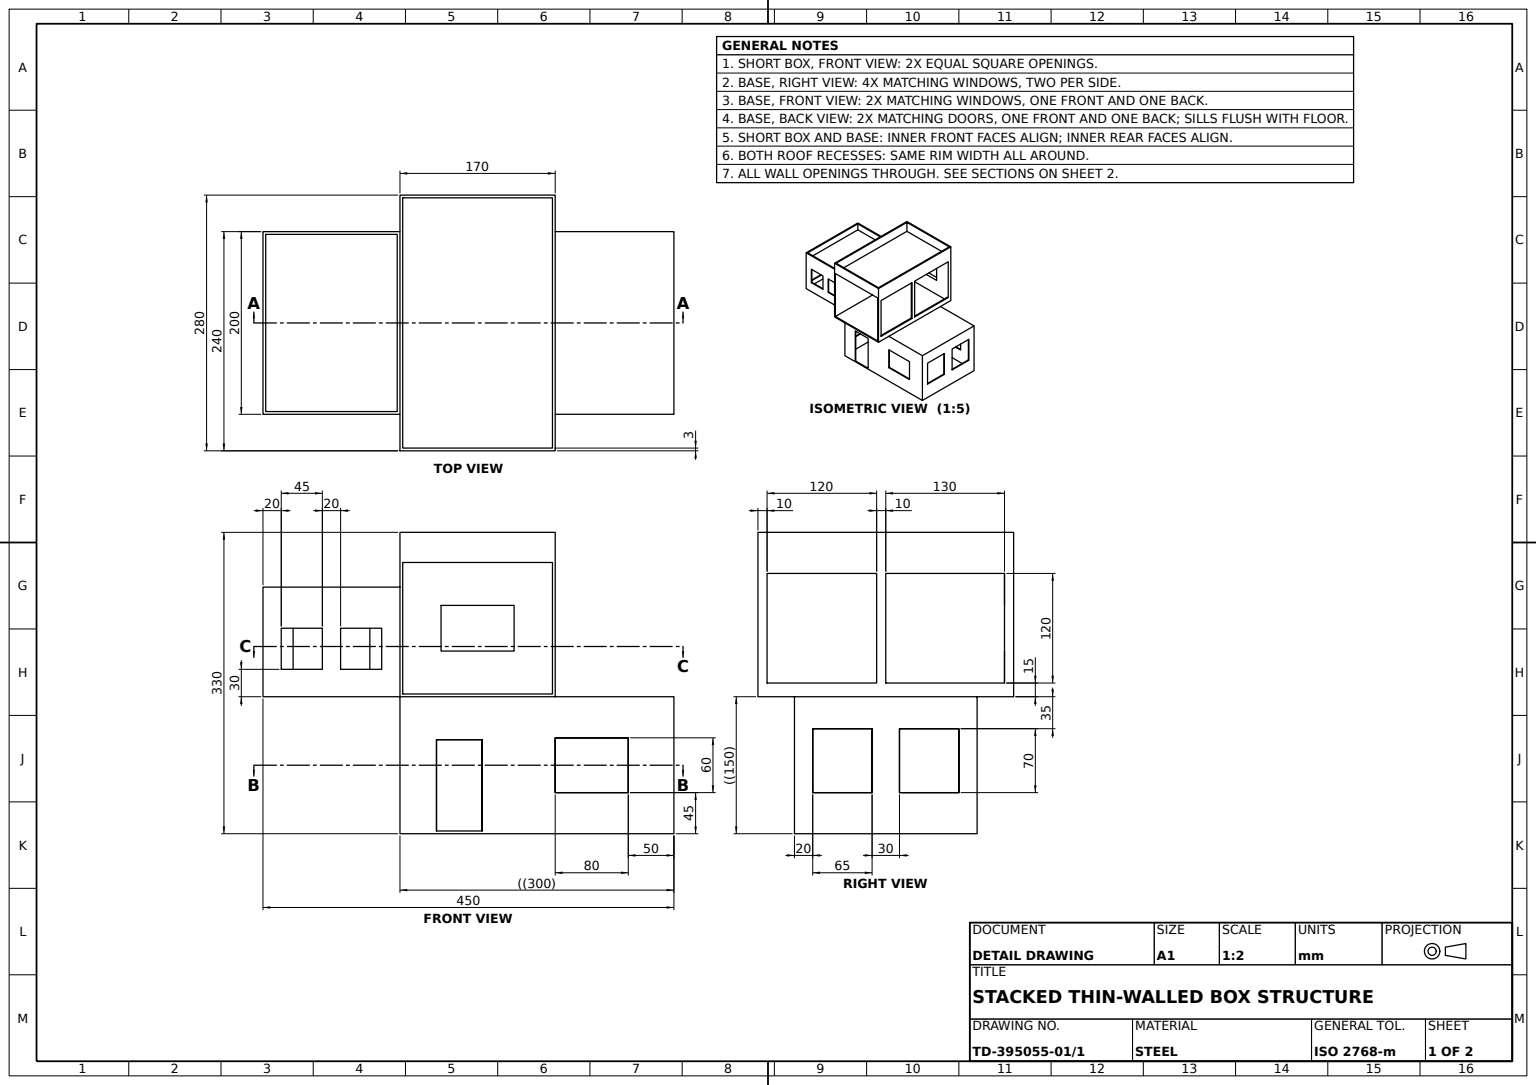
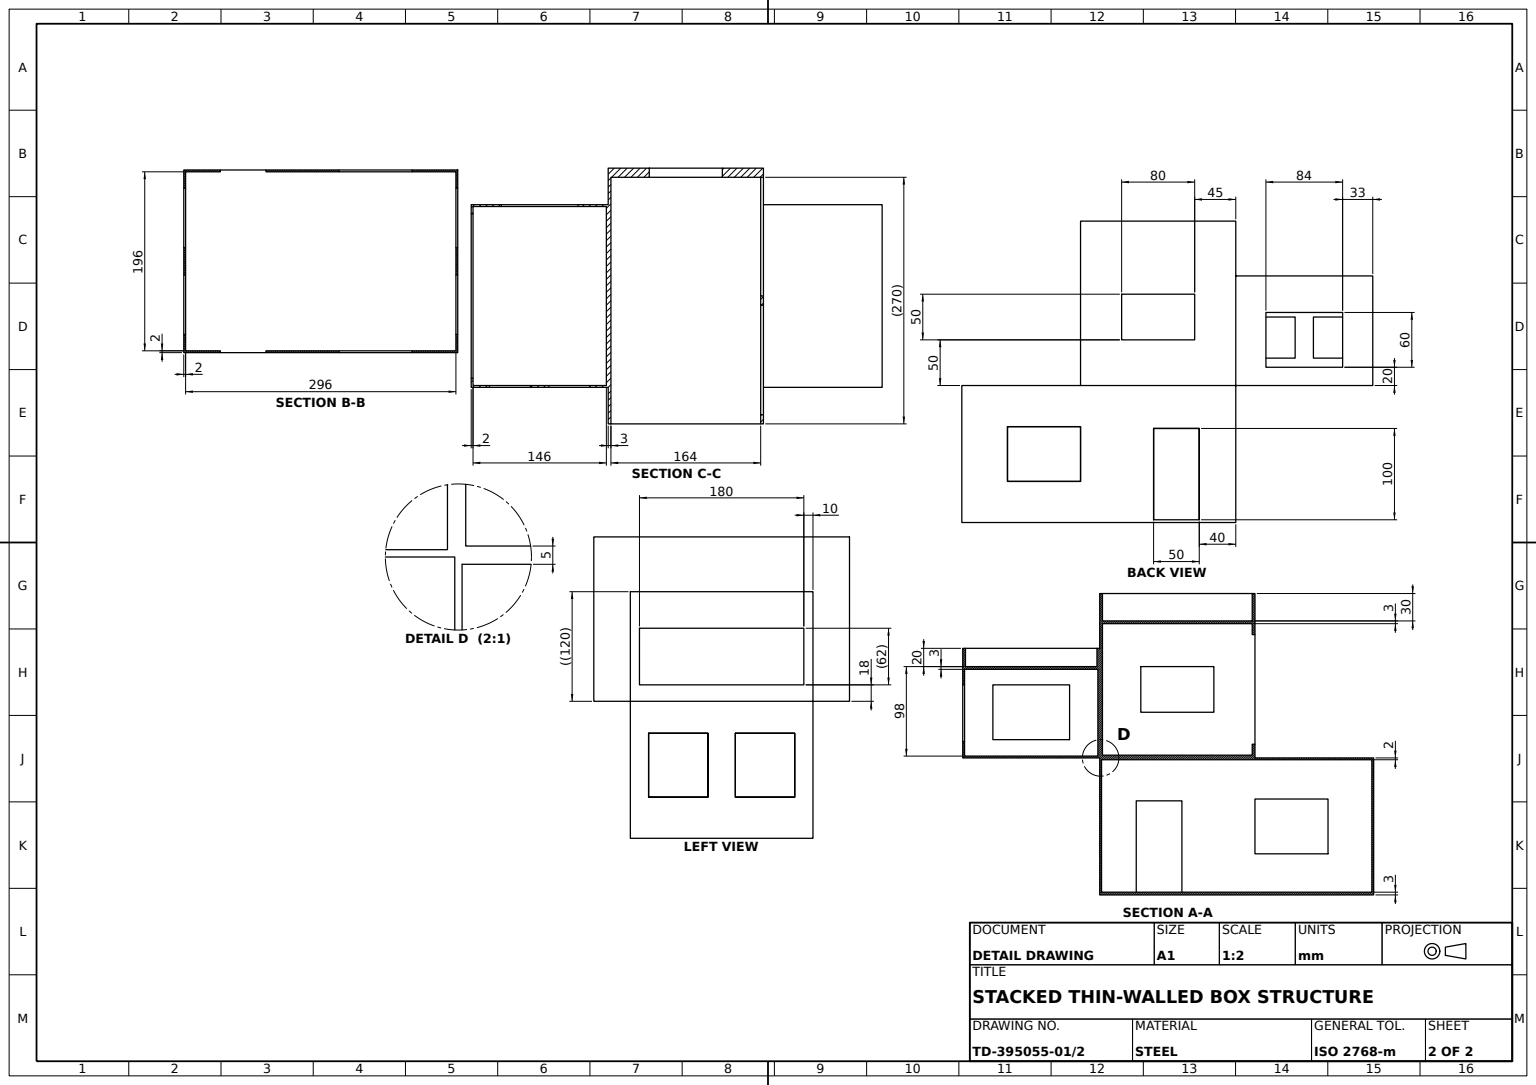
from build123d import *

# Parameters (mm, degrees)
GROUND_FLOOR_FOOTPRINT_SKETCH_W     = 300
GROUND_FLOOR_FOOTPRINT_SKETCH_H     = 200
GROUND_FLOOR_BLOCK_DEPTH            = 150
GROUND_FLOOR_DOOR_SKETCH_W          = 50
GROUND_FLOOR_DOOR_SKETCH_H          = 100
GROUND_FLOOR_DOOR_OPENING_DEPTH     = 210
GROUND_FLOOR_INTERIOR_POCKET_REACH  = 392.512
GROUND_FLOOR_INTERIOR_SKETCH_W      = 296
GROUND_FLOOR_INTERIOR_SKETCH_H      = 196
GROUND_FLOOR_SLAB_SKETCH_W          = 300
GROUND_FLOOR_SLAB_SKETCH_H          = 200
GROUND_FLOOR_SLAB_DEPTH             = 2
GROUND_FLOOR_WINDOW_SKETCH_W        = 80
GROUND_FLOOR_WINDOW_SKETCH_H        = 60
GROUND_FLOOR_WINDOW_DEPTH           = 312
GROUND_FLOOR_SIDE_WINDOWS_SKETCH_W  = 65
GROUND_FLOOR_SIDE_WINDOWS_SKETCH_H  = 70
GROUND_FLOOR_SIDE_WINDOWS_DEPTH     = 312
FIRST_FLOOR_FOOTPRINT_SKETCH_W      = 150
FIRST_FLOOR_FOOTPRINT_SKETCH_H      = 200
FIRST_FLOOR_BLOCK_DEPTH             = 100
FIRST_FLOOR_INTERIOR_SKETCH_W       = 146
FIRST_FLOOR_INTERIOR_SKETCH_H       = 196
FIRST_FLOOR_INTERIOR_POCKET_DEPTH   = 98
FIRST_FLOOR_SLAB_SKETCH_W           = 150
FIRST_FLOOR_SLAB_SKETCH_H           = 200
FIRST_FLOOR_SLAB_DEPTH              = 3
FIRST_FLOOR_DOOR_SKETCH_W           = 180
FIRST_FLOOR_DOOR_SKETCH_H           = 62
FIRST_FLOOR_DOOR_OPENING_DEPTH      = 23
FIRST_FLOOR_TWIN_WINDOWS_SKETCH_W   = 45
FIRST_FLOOR_TWIN_WINDOWS_SKETCH_H   = 45
FIRST_FLOOR_TWIN_WINDOWS_DEPTH      = 23
FIRST_FLOOR_WINDOW_SKETCH_W         = 84
FIRST_FLOOR_WINDOW_SKETCH_H         = 60
FIRST_FLOOR_WINDOW_DEPTH            = 23
FIRST_FLOOR_PARAPET_FRONT_SKETCH_W  = 200
FIRST_FLOOR_PARAPET_FRONT_SKETCH_H  = 20
FIRST_FLOOR_PARAPET_FRONT_DEPTH     = 3
FIRST_FLOOR_PARAPET_SIDE_1_SKETCH_W = 150
FIRST_FLOOR_PARAPET_SIDE_1_SKETCH_H = 20
FIRST_FLOOR_PARAPET_SIDE_1_DEPTH    = 3
FIRST_FLOOR_PARAPET_SIDE_2_SKETCH_W = 150
FIRST_FLOOR_PARAPET_SIDE_2_SKETCH_H = 20
FIRST_FLOOR_PARAPET_SIDE_2_DEPTH    = 3
FIRST_FLOOR_PARAPET_REAR_SKETCH_W   = 197
FIRST_FLOOR_PARAPET_REAR_SKETCH_H   = 20
FIRST_FLOOR_PARAPET_REAR_DEPTH      = 3
UPPER_FLOOR_BLOCK_DEPTH             = 40
UPPER_FLOOR_BLOCK_DEPTH_BACK        = 240
UPPER_FLOOR_PROFILE_SKETCH_W        = 170
UPPER_FLOOR_PROFILE_SKETCH_H        = 150
UPPER_FLOOR_INTERIOR_SKETCH_W       = 164
UPPER_FLOOR_INTERIOR_SKETCH_H       = 144
UPPER_FLOOR_INTERIOR_POCKET_DEPTH   = 270
UPPER_FLOOR_OPENING_1_SKETCH_W      = 120
UPPER_FLOOR_OPENING_1_SKETCH_H      = 120
UPPER_FLOOR_OPENING_1_DEPTH         = 100
UPPER_FLOOR_OPENING_2_SKETCH_W      = 130
UPPER_FLOOR_OPENING_2_SKETCH_H      = 120
UPPER_FLOOR_OPENING_2_DEPTH         = 100
UPPER_FLOOR_WINDOW_SKETCH_W         = 80
UPPER_FLOOR_WINDOW_SKETCH_H         = 50
UPPER_FLOOR_WINDOW_DEPTH            = 100
UPPER_FLOOR_PARAPET_FRONT_SKETCH_W  = 170
UPPER_FLOOR_PARAPET_FRONT_SKETCH_H  = 30
UPPER_FLOOR_PARAPET_FRONT_DEPTH     = 3
UPPER_FLOOR_PARAPET_SIDE_1_SKETCH_W = 277
UPPER_FLOOR_PARAPET_SIDE_1_SKETCH_H = 30
UPPER_FLOOR_PARAPET_SIDE_1_DEPTH    = 3
UPPER_FLOOR_PARAPET_SIDE_2_SKETCH_W = 170
UPPER_FLOOR_PARAPET_SIDE_2_SKETCH_H = 30
UPPER_FLOOR_PARAPET_SIDE_2_DEPTH    = 3
UPPER_FLOOR_PARAPET_REAR_SKETCH_W   = 274
UPPER_FLOOR_PARAPET_REAR_SKETCH_H   = 30
UPPER_FLOOR_PARAPET_REAR_DEPTH      = 3


with BuildPart() as part:
    # Ground Floor Footprint Sketch → Ground Floor Block (new body)
    with BuildSketch(Plane(origin=(0, 0, 0), x_dir=(1, 0, 0), z_dir=(0, 1, 0))):
        with Locations((150, 100)):
            Rectangle(GROUND_FLOOR_FOOTPRINT_SKETCH_W, GROUND_FLOOR_FOOTPRINT_SKETCH_H)
    extrude(amount=GROUND_FLOOR_BLOCK_DEPTH)

    # Ground Floor Door Sketch → Ground Floor Door Opening (cut)
    with BuildSketch(Plane.XY):
        with Locations((65, 53)):
            Rectangle(GROUND_FLOOR_DOOR_SKETCH_W, GROUND_FLOOR_DOOR_SKETCH_H)
    extrude(amount=-GROUND_FLOOR_DOOR_OPENING_DEPTH, mode=Mode.SUBTRACT)

    # Ground Floor Interior Pocket: up to this face of the body (flat: up to its plane)
    ground_floor_interior_pocket_end = Plane(part.part.faces().sort_by_distance((65, 3, -100))[0])
    # Ground Floor Interior Sketch → Ground Floor Interior Pocket (cut, up to the picked face)
    with BuildSketch(Plane(origin=(0, 150, 0), x_dir=(1, 0, 0), z_dir=(0, 1, 0)), mode=Mode.PRIVATE) as ground_floor_interior_pocket_sk1:
        with Locations((150, 100)):
            Rectangle(GROUND_FLOOR_INTERIOR_SKETCH_W, GROUND_FLOOR_INTERIOR_SKETCH_H)
    ground_floor_interior_pocket_tool1 = split(extrude(ground_floor_interior_pocket_sk1.sketch, amount=-GROUND_FLOOR_INTERIOR_POCKET_REACH, mode=Mode.PRIVATE), bisect_by=ground_floor_interior_pocket_end, keep=Keep.BOTH, mode=Mode.PRIVATE)
    add(ground_floor_interior_pocket_tool1.solids().sort_by(Axis((150, 150, -100), (0, -1, 0)))[0], mode=Mode.SUBTRACT)

    # Ground Floor Slab Sketch → Ground Floor Slab (add)
    with BuildSketch(Plane(origin=(0, 150, 0), x_dir=(1, 0, 0), z_dir=(0, 1, 0))):
        with Locations((150, 100)):
            Rectangle(GROUND_FLOOR_SLAB_SKETCH_W, GROUND_FLOOR_SLAB_SKETCH_H)
    extrude(amount=-GROUND_FLOOR_SLAB_DEPTH)

    # Ground Floor Window Sketch → Ground Floor Window (cut)
    with BuildSketch(Plane.XY):
        with Locations((210, 75)):
            Rectangle(GROUND_FLOOR_WINDOW_SKETCH_W, GROUND_FLOOR_WINDOW_SKETCH_H)
    extrude(amount=-GROUND_FLOOR_WINDOW_DEPTH, mode=Mode.SUBTRACT)

    # Ground Floor Side Windows Sketch → Ground Floor Side Windows (cut)
    with BuildSketch(Plane(origin=(300, 0, 0), x_dir=(0, 0, -1), z_dir=(1, 0, 0))):
        with Locations((52.5, 80)):
            Rectangle(GROUND_FLOOR_SIDE_WINDOWS_SKETCH_W, GROUND_FLOOR_SIDE_WINDOWS_SKETCH_H)
        with Locations((147.5, 80)):
            Rectangle(GROUND_FLOOR_SIDE_WINDOWS_SKETCH_W, GROUND_FLOOR_SIDE_WINDOWS_SKETCH_H)
    extrude(amount=-GROUND_FLOOR_SIDE_WINDOWS_DEPTH, mode=Mode.SUBTRACT)



with BuildPart() as body_2:
    # First Floor Footprint Sketch → First Floor Block (new body)
    with BuildSketch(Plane(origin=(0, 150, 0), x_dir=(1, 0, 0), z_dir=(0, 1, 0))):
        with Locations((-75, 100)):
            Rectangle(FIRST_FLOOR_FOOTPRINT_SKETCH_W, FIRST_FLOOR_FOOTPRINT_SKETCH_H)
    extrude(amount=FIRST_FLOOR_BLOCK_DEPTH)

    # First Floor Interior Sketch → First Floor Interior Pocket (cut)
    with BuildSketch(Plane(origin=(0, 250, 0), x_dir=(1, 0, 0), z_dir=(0, 1, 0))):
        with Locations((-75, 100)):
            Rectangle(FIRST_FLOOR_INTERIOR_SKETCH_W, FIRST_FLOOR_INTERIOR_SKETCH_H)
    extrude(amount=-FIRST_FLOOR_INTERIOR_POCKET_DEPTH, mode=Mode.SUBTRACT)

    # First Floor Slab Sketch → First Floor Slab (add)
    with BuildSketch(Plane(origin=(0, 250, 0), x_dir=(1, 0, 0), z_dir=(0, 1, 0))):
        with Locations((-75, 100)):
            Rectangle(FIRST_FLOOR_SLAB_SKETCH_W, FIRST_FLOOR_SLAB_SKETCH_H)
    extrude(amount=-FIRST_FLOOR_SLAB_DEPTH)

    # First Floor Door Sketch → First Floor Door Opening (cut)
    with BuildSketch(Plane.ZY.offset(150)):
        with Locations((-100, 199)):
            Rectangle(FIRST_FLOOR_DOOR_SKETCH_W, FIRST_FLOOR_DOOR_SKETCH_H)
    extrude(amount=-FIRST_FLOOR_DOOR_OPENING_DEPTH, mode=Mode.SUBTRACT)

    # First Floor Twin Windows Sketch → First Floor Twin Windows (cut)
    with BuildSketch(Plane.XY):
        with Locations((-107.5, 202.5)):
            Rectangle(FIRST_FLOOR_TWIN_WINDOWS_SKETCH_W, FIRST_FLOOR_TWIN_WINDOWS_SKETCH_H)
        with Locations((-42.5, 202.5)):
            Rectangle(FIRST_FLOOR_TWIN_WINDOWS_SKETCH_W, FIRST_FLOOR_TWIN_WINDOWS_SKETCH_H)
    extrude(amount=-FIRST_FLOOR_TWIN_WINDOWS_DEPTH, mode=Mode.SUBTRACT)

    # First Floor Window Sketch → First Floor Window (cut)
    with BuildSketch(Plane(origin=(0, 0, -200), x_dir=(-1, 0, 0), z_dir=(0, 0, -1))):
        with Locations((75, 200)):
            Rectangle(FIRST_FLOOR_WINDOW_SKETCH_W, FIRST_FLOOR_WINDOW_SKETCH_H)
    extrude(amount=-FIRST_FLOOR_WINDOW_DEPTH, mode=Mode.SUBTRACT)

    # First Floor Parapet Front Sketch → First Floor Parapet Front (add)
    with BuildSketch(Plane.ZY.offset(150)):
        with Locations((-100, 260)):
            Rectangle(FIRST_FLOOR_PARAPET_FRONT_SKETCH_W, FIRST_FLOOR_PARAPET_FRONT_SKETCH_H)
    extrude(amount=-FIRST_FLOOR_PARAPET_FRONT_DEPTH)

    # First Floor Parapet Side 1 Sketch → First Floor Parapet Side 1 (add)
    with BuildSketch(Plane(origin=(0, 0, -200), x_dir=(-1, 0, 0), z_dir=(0, 0, -1))):
        with Locations((75, 260)):
            Rectangle(FIRST_FLOOR_PARAPET_SIDE_1_SKETCH_W, FIRST_FLOOR_PARAPET_SIDE_1_SKETCH_H)
    extrude(amount=-FIRST_FLOOR_PARAPET_SIDE_1_DEPTH)

    # First Floor Parapet Side 2 Sketch → First Floor Parapet Side 2 (add)
    with BuildSketch(Plane.XY):
        with Locations((-75, 260)):
            Rectangle(FIRST_FLOOR_PARAPET_SIDE_2_SKETCH_W, FIRST_FLOOR_PARAPET_SIDE_2_SKETCH_H)
    extrude(amount=-FIRST_FLOOR_PARAPET_SIDE_2_DEPTH)

    # First Floor Parapet Rear Sketch → First Floor Parapet Rear (add)
    with BuildSketch(Plane(origin=(0, 0, 0), x_dir=(0, 0, -1), z_dir=(1, 0, 0))):
        with Locations((98.5, 260)):
            Rectangle(FIRST_FLOOR_PARAPET_REAR_SKETCH_W, FIRST_FLOOR_PARAPET_REAR_SKETCH_H)
    extrude(amount=-FIRST_FLOOR_PARAPET_REAR_DEPTH)


with BuildPart() as part_1:
    add(part.part)

    add(body_2.part)  # Upper Floor Block merges body 2
    # Upper Floor Profile Sketch → Upper Floor Block (add, two sides: drawn at the far end of the back side and taken through both)
    with BuildSketch(Plane.XY.offset(-UPPER_FLOOR_BLOCK_DEPTH_BACK)):
        with Locations((85, 225)):
            Rectangle(UPPER_FLOOR_PROFILE_SKETCH_W, UPPER_FLOOR_PROFILE_SKETCH_H)
    extrude(amount=UPPER_FLOOR_BLOCK_DEPTH + UPPER_FLOOR_BLOCK_DEPTH_BACK)

    # Upper Floor Interior Sketch → Upper Floor Interior Pocket (cut)
    with BuildSketch(Plane.XY.offset(40)):
        with Locations((85, 225)):
            Rectangle(UPPER_FLOOR_INTERIOR_SKETCH_W, UPPER_FLOOR_INTERIOR_SKETCH_H)
    extrude(amount=-UPPER_FLOOR_INTERIOR_POCKET_DEPTH, mode=Mode.SUBTRACT)

    # Upper Floor Opening 1 Sketch → Upper Floor Opening 1 (cut)
    with BuildSketch(Plane(origin=(170, 0, 0), x_dir=(0, 0, -1), z_dir=(1, 0, 0))):
        with Locations((30, 225)):
            Rectangle(UPPER_FLOOR_OPENING_1_SKETCH_W, UPPER_FLOOR_OPENING_1_SKETCH_H)
    extrude(amount=-UPPER_FLOOR_OPENING_1_DEPTH, mode=Mode.SUBTRACT)

    # Upper Floor Opening 2 Sketch → Upper Floor Opening 2 (cut)
    with BuildSketch(Plane(origin=(170, 0, 0), x_dir=(0, 0, -1), z_dir=(1, 0, 0))):
        with Locations((165, 225)):
            Rectangle(UPPER_FLOOR_OPENING_2_SKETCH_W, UPPER_FLOOR_OPENING_2_SKETCH_H)
    extrude(amount=-UPPER_FLOOR_OPENING_2_DEPTH, mode=Mode.SUBTRACT)

    # Upper Floor Window Sketch → Upper Floor Window (cut)
    with BuildSketch(Plane(origin=(0, 0, -240), x_dir=(-1, 0, 0), z_dir=(0, 0, -1))):
        with Locations((-85, 225)):
            Rectangle(UPPER_FLOOR_WINDOW_SKETCH_W, UPPER_FLOOR_WINDOW_SKETCH_H)
    extrude(amount=-UPPER_FLOOR_WINDOW_DEPTH, mode=Mode.SUBTRACT)

    # Upper Floor Parapet Front Sketch → Upper Floor Parapet Front (add)
    with BuildSketch(Plane(origin=(0, 0, -240), x_dir=(-1, 0, 0), z_dir=(0, 0, -1))):
        with Locations((-85, 315)):
            Rectangle(UPPER_FLOOR_PARAPET_FRONT_SKETCH_W, UPPER_FLOOR_PARAPET_FRONT_SKETCH_H)
    extrude(amount=-UPPER_FLOOR_PARAPET_FRONT_DEPTH)

    # Upper Floor Parapet Side 1 Sketch → Upper Floor Parapet Side 1 (add)
    with BuildSketch(Plane(origin=(170, 0, 0), x_dir=(0, 0, -1), z_dir=(1, 0, 0))):
        with Locations((98.5, 315)):
            Rectangle(UPPER_FLOOR_PARAPET_SIDE_1_SKETCH_W, UPPER_FLOOR_PARAPET_SIDE_1_SKETCH_H)
    extrude(amount=-UPPER_FLOOR_PARAPET_SIDE_1_DEPTH)

    # Upper Floor Parapet Side 2 Sketch → Upper Floor Parapet Side 2 (add)
    with BuildSketch(Plane.XY.offset(40)):
        with Locations((85, 315)):
            Rectangle(UPPER_FLOOR_PARAPET_SIDE_2_SKETCH_W, UPPER_FLOOR_PARAPET_SIDE_2_SKETCH_H)
    extrude(amount=-UPPER_FLOOR_PARAPET_SIDE_2_DEPTH)

    # Upper Floor Parapet Rear Sketch → Upper Floor Parapet Rear (add)
    with BuildSketch(Plane.ZY):
        with Locations((-100, 315)):
            Rectangle(UPPER_FLOOR_PARAPET_REAR_SKETCH_W, UPPER_FLOOR_PARAPET_REAR_SKETCH_H)
    extrude(amount=-UPPER_FLOOR_PARAPET_REAR_DEPTH)


solid = part_1.part
